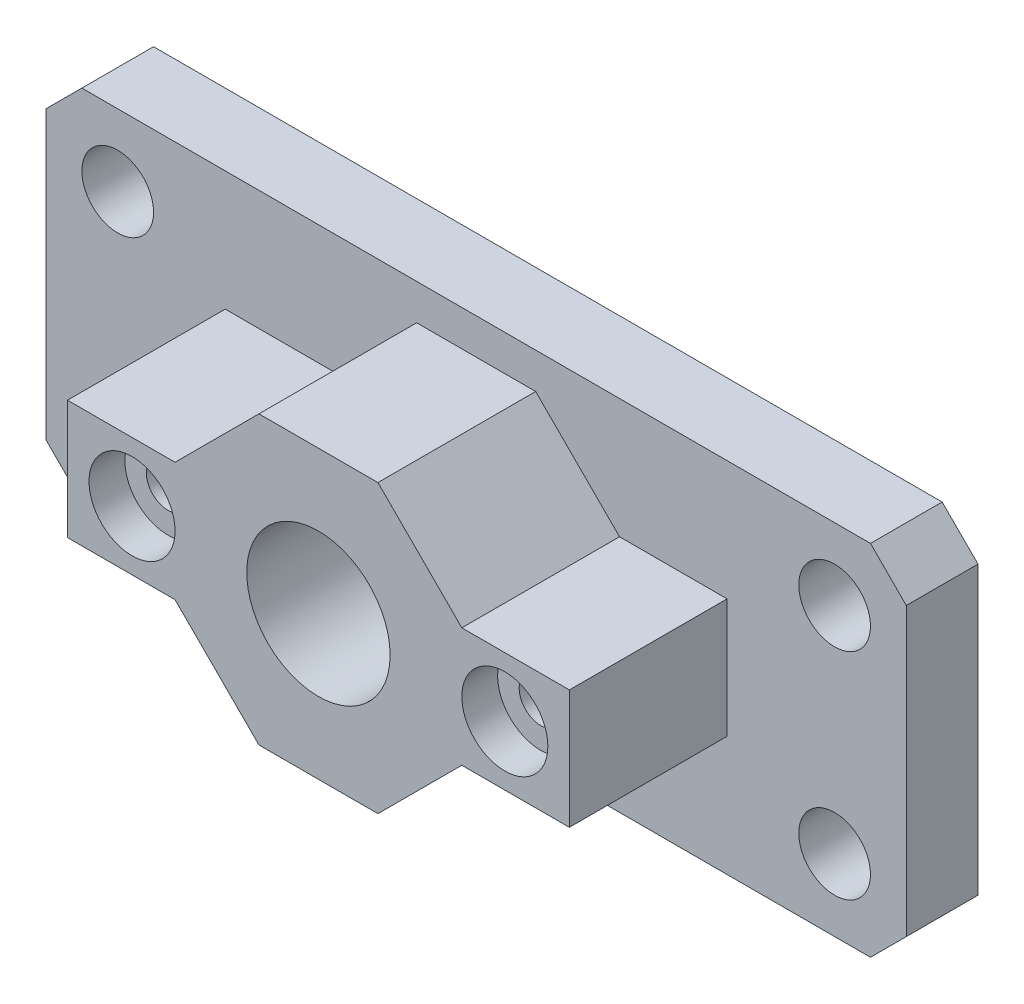
ISO-10303-21;
HEADER;
FILE_DESCRIPTION(('STEP AP214'),'2;1');
FILE_NAME('part.step','',(''),(''),'','','');
FILE_SCHEMA(('AUTOMOTIVE_DESIGN { 1 0 10303 214 1 1 1 1 }'));
ENDSEC;
DATA;
#1=APPLICATION_CONTEXT('core data for automotive mechanical design processes');
#2=APPLICATION_PROTOCOL_DEFINITION('international standard','automotive_design',2000,#1);
#3=PRODUCT_CONTEXT('',#1,'mechanical');
#4=PRODUCT('Part','Part','',(#3));
#5=PRODUCT_RELATED_PRODUCT_CATEGORY('part','',(#4));
#6=PRODUCT_DEFINITION_FORMATION('','',#4);
#7=PRODUCT_DEFINITION_CONTEXT('part definition',#1,'design');
#8=PRODUCT_DEFINITION('design','',#6,#7);
#9=PRODUCT_DEFINITION_SHAPE('','',#8);
#10=(LENGTH_UNIT() NAMED_UNIT(*) SI_UNIT(.MILLI.,.METRE.));
#11=(NAMED_UNIT(*) PLANE_ANGLE_UNIT() SI_UNIT($,.RADIAN.));
#12=(NAMED_UNIT(*) SI_UNIT($,.STERADIAN.) SOLID_ANGLE_UNIT());
#13=UNCERTAINTY_MEASURE_WITH_UNIT(LENGTH_MEASURE(1.E-05),#10,'distance_accuracy_value','');
#14=(GEOMETRIC_REPRESENTATION_CONTEXT(3) GLOBAL_UNCERTAINTY_ASSIGNED_CONTEXT((#13)) GLOBAL_UNIT_ASSIGNED_CONTEXT((#10,
#11,#12)) REPRESENTATION_CONTEXT('',''));
#15=CARTESIAN_POINT('',(0.,0.,0.));
#16=DIRECTION('',(0.,0.,1.));
#17=DIRECTION('',(1.,0.,0.));
#18=AXIS2_PLACEMENT_3D('',#15,#16,#17);
#19=CARTESIAN_POINT('',(60.,25.,10.));
#20=DIRECTION('',(-1.,0.,0.));
#21=DIRECTION('',(0.,-1.,0.));
#22=AXIS2_PLACEMENT_3D('',#19,#20,#21);
#23=PLANE('',#22);
#24=DIRECTION('',(0.,1.,0.));
#25=VECTOR('',#24,1.);
#26=CARTESIAN_POINT('',(60.,25.,10.));
#27=LINE('',#26,#25);
#28=CARTESIAN_POINT('',(60.,-20.,10.));
#29=VERTEX_POINT('',#28);
#30=CARTESIAN_POINT('',(60.,20.,10.));
#31=VERTEX_POINT('',#30);
#32=EDGE_CURVE('E216',#29,#31,#27,.T.);
#33=ORIENTED_EDGE('',*,*,#32,.F.);
#34=DIRECTION('',(0.,0.,-1.));
#35=VECTOR('',#34,1.);
#36=CARTESIAN_POINT('',(60.,-20.,10.));
#37=LINE('',#36,#35);
#38=CARTESIAN_POINT('',(60.,-20.,0.));
#39=VERTEX_POINT('',#38);
#40=EDGE_CURVE('E249',#29,#39,#37,.T.);
#41=ORIENTED_EDGE('',*,*,#40,.T.);
#42=DIRECTION('',(0.,1.,0.));
#43=VECTOR('',#42,1.);
#44=CARTESIAN_POINT('',(60.,25.,0.));
#45=LINE('',#44,#43);
#46=CARTESIAN_POINT('',(60.,20.,0.));
#47=VERTEX_POINT('',#46);
#48=EDGE_CURVE('E210',#39,#47,#45,.T.);
#49=ORIENTED_EDGE('',*,*,#48,.T.);
#50=DIRECTION('',(0.,0.,1.));
#51=VECTOR('',#50,1.);
#52=CARTESIAN_POINT('',(60.,20.,10.));
#53=LINE('',#52,#51);
#54=EDGE_CURVE('E227',#47,#31,#53,.T.);
#55=ORIENTED_EDGE('',*,*,#54,.T.);
#56=EDGE_LOOP('',(#33,#41,#49,#55));
#57=FACE_BOUND('',#56,.T.);
#58=ADVANCED_FACE('F41',(#57),#23,.F.);
#59=CARTESIAN_POINT('',(-60.,25.,10.));
#60=DIRECTION('',(0.,-1.,0.));
#61=DIRECTION('',(0.,0.,-1.));
#62=AXIS2_PLACEMENT_3D('',#59,#60,#61);
#63=PLANE('',#62);
#64=DIRECTION('',(-1.,0.,0.));
#65=VECTOR('',#64,1.);
#66=CARTESIAN_POINT('',(-60.,25.,0.));
#67=LINE('',#66,#65);
#68=CARTESIAN_POINT('',(55.,25.,0.));
#69=VERTEX_POINT('',#68);
#70=CARTESIAN_POINT('',(-55.,25.,0.));
#71=VERTEX_POINT('',#70);
#72=EDGE_CURVE('E209',#69,#71,#67,.T.);
#73=ORIENTED_EDGE('',*,*,#72,.T.);
#74=DIRECTION('',(0.,0.,1.));
#75=VECTOR('',#74,1.);
#76=CARTESIAN_POINT('',(-55.,25.,10.));
#77=LINE('',#76,#75);
#78=CARTESIAN_POINT('',(-55.,25.,10.));
#79=VERTEX_POINT('',#78);
#80=EDGE_CURVE('E11',#71,#79,#77,.T.);
#81=ORIENTED_EDGE('',*,*,#80,.T.);
#82=DIRECTION('',(-1.,0.,0.));
#83=VECTOR('',#82,1.);
#84=CARTESIAN_POINT('',(-60.,25.,10.));
#85=LINE('',#84,#83);
#86=CARTESIAN_POINT('',(55.,25.,10.));
#87=VERTEX_POINT('',#86);
#88=EDGE_CURVE('E218',#87,#79,#85,.T.);
#89=ORIENTED_EDGE('',*,*,#88,.F.);
#90=DIRECTION('',(0.,0.,-1.));
#91=VECTOR('',#90,1.);
#92=CARTESIAN_POINT('',(55.,25.,10.));
#93=LINE('',#92,#91);
#94=EDGE_CURVE('E49',#87,#69,#93,.T.);
#95=ORIENTED_EDGE('',*,*,#94,.T.);
#96=EDGE_LOOP('',(#73,#81,#89,#95));
#97=FACE_BOUND('',#96,.T.);
#98=ADVANCED_FACE('F278',(#97),#63,.F.);
#99=CARTESIAN_POINT('',(-60.,25.,10.));
#100=DIRECTION('',(1.,0.,0.));
#101=DIRECTION('',(0.,1.,0.));
#102=AXIS2_PLACEMENT_3D('',#99,#100,#101);
#103=PLANE('',#102);
#104=DIRECTION('',(0.,-1.,0.));
#105=VECTOR('',#104,1.);
#106=CARTESIAN_POINT('',(-60.,25.,0.));
#107=LINE('',#106,#105);
#108=CARTESIAN_POINT('',(-60.,20.,0.));
#109=VERTEX_POINT('',#108);
#110=CARTESIAN_POINT('',(-60.,-20.,0.));
#111=VERTEX_POINT('',#110);
#112=EDGE_CURVE('E228',#109,#111,#107,.T.);
#113=ORIENTED_EDGE('',*,*,#112,.T.);
#114=DIRECTION('',(0.,0.,1.));
#115=VECTOR('',#114,1.);
#116=CARTESIAN_POINT('',(-60.,-20.,10.));
#117=LINE('',#116,#115);
#118=CARTESIAN_POINT('',(-60.,-20.,10.));
#119=VERTEX_POINT('',#118);
#120=EDGE_CURVE('E60',#111,#119,#117,.T.);
#121=ORIENTED_EDGE('',*,*,#120,.T.);
#122=DIRECTION('',(0.,-1.,0.));
#123=VECTOR('',#122,1.);
#124=CARTESIAN_POINT('',(-60.,25.,10.));
#125=LINE('',#124,#123);
#126=CARTESIAN_POINT('',(-60.,20.,10.));
#127=VERTEX_POINT('',#126);
#128=EDGE_CURVE('E225',#127,#119,#125,.T.);
#129=ORIENTED_EDGE('',*,*,#128,.F.);
#130=DIRECTION('',(0.,0.,-1.));
#131=VECTOR('',#130,1.);
#132=CARTESIAN_POINT('',(-60.,20.,10.));
#133=LINE('',#132,#131);
#134=EDGE_CURVE('E275',#127,#109,#133,.T.);
#135=ORIENTED_EDGE('',*,*,#134,.T.);
#136=EDGE_LOOP('',(#113,#121,#129,#135));
#137=FACE_BOUND('',#136,.T.);
#138=ADVANCED_FACE('F292',(#137),#103,.F.);
#139=CARTESIAN_POINT('',(-60.,-25.,10.));
#140=DIRECTION('',(0.,1.,0.));
#141=DIRECTION('',(0.,0.,1.));
#142=AXIS2_PLACEMENT_3D('',#139,#140,#141);
#143=PLANE('',#142);
#144=DIRECTION('',(1.,0.,0.));
#145=VECTOR('',#144,1.);
#146=CARTESIAN_POINT('',(-60.,-25.,0.));
#147=LINE('',#146,#145);
#148=CARTESIAN_POINT('',(-55.,-25.,0.));
#149=VERTEX_POINT('',#148);
#150=CARTESIAN_POINT('',(55.,-25.,0.));
#151=VERTEX_POINT('',#150);
#152=EDGE_CURVE('E219',#149,#151,#147,.T.);
#153=ORIENTED_EDGE('',*,*,#152,.T.);
#154=DIRECTION('',(0.,0.,1.));
#155=VECTOR('',#154,1.);
#156=CARTESIAN_POINT('',(55.,-25.,10.));
#157=LINE('',#156,#155);
#158=CARTESIAN_POINT('',(55.,-25.,10.));
#159=VERTEX_POINT('',#158);
#160=EDGE_CURVE('E263',#151,#159,#157,.T.);
#161=ORIENTED_EDGE('',*,*,#160,.T.);
#162=DIRECTION('',(1.,0.,0.));
#163=VECTOR('',#162,1.);
#164=CARTESIAN_POINT('',(-60.,-25.,10.));
#165=LINE('',#164,#163);
#166=CARTESIAN_POINT('',(-55.,-25.,10.));
#167=VERTEX_POINT('',#166);
#168=EDGE_CURVE('E221',#167,#159,#165,.T.);
#169=ORIENTED_EDGE('',*,*,#168,.F.);
#170=DIRECTION('',(0.,0.,-1.));
#171=VECTOR('',#170,1.);
#172=CARTESIAN_POINT('',(-55.,-25.,10.));
#173=LINE('',#172,#171);
#174=EDGE_CURVE('E257',#167,#149,#173,.T.);
#175=ORIENTED_EDGE('',*,*,#174,.T.);
#176=EDGE_LOOP('',(#153,#161,#169,#175));
#177=FACE_BOUND('',#176,.T.);
#178=ADVANCED_FACE('F298',(#177),#143,.F.);
#179=CARTESIAN_POINT('',(0.,0.,10.));
#180=DIRECTION('',(0.,0.,1.));
#181=DIRECTION('',(1.,0.,0.));
#182=AXIS2_PLACEMENT_3D('',#179,#180,#181);
#183=PLANE('',#182);
#184=CARTESIAN_POINT('',(50.,-15.,10.));
#185=DIRECTION('',(0.,0.,1.));
#186=DIRECTION('',(1.,0.,0.));
#187=AXIS2_PLACEMENT_3D('',#184,#185,#186);
#188=CIRCLE('',#187,5.);
#189=CARTESIAN_POINT('',(55.,-15.,10.));
#190=VERTEX_POINT('',#189);
#191=EDGE_CURVE('E643',#190,#190,#188,.T.);
#192=ORIENTED_EDGE('',*,*,#191,.F.);
#193=EDGE_LOOP('',(#192));
#194=FACE_BOUND('',#193,.T.);
#195=CARTESIAN_POINT('',(-50.,15.,10.));
#196=DIRECTION('',(0.,0.,1.));
#197=DIRECTION('',(1.,0.,0.));
#198=AXIS2_PLACEMENT_3D('',#195,#196,#197);
#199=CIRCLE('',#198,5.);
#200=CARTESIAN_POINT('',(-45.,15.,10.));
#201=VERTEX_POINT('',#200);
#202=EDGE_CURVE('E642',#201,#201,#199,.T.);
#203=ORIENTED_EDGE('',*,*,#202,.F.);
#204=EDGE_LOOP('',(#203));
#205=FACE_BOUND('',#204,.T.);
#206=CARTESIAN_POINT('',(-50.,-15.,10.));
#207=DIRECTION('',(0.,0.,1.));
#208=DIRECTION('',(1.,0.,0.));
#209=AXIS2_PLACEMENT_3D('',#206,#207,#208);
#210=CIRCLE('',#209,5.);
#211=CARTESIAN_POINT('',(-45.,-15.,10.));
#212=VERTEX_POINT('',#211);
#213=EDGE_CURVE('E647',#212,#212,#210,.T.);
#214=ORIENTED_EDGE('',*,*,#213,.F.);
#215=EDGE_LOOP('',(#214));
#216=FACE_BOUND('',#215,.T.);
#217=CARTESIAN_POINT('',(50.,15.,10.));
#218=DIRECTION('',(0.,0.,1.));
#219=DIRECTION('',(1.,0.,0.));
#220=AXIS2_PLACEMENT_3D('',#217,#218,#219);
#221=CIRCLE('',#220,5.);
#222=CARTESIAN_POINT('',(55.,15.,10.));
#223=VERTEX_POINT('',#222);
#224=EDGE_CURVE('E236',#223,#223,#221,.T.);
#225=ORIENTED_EDGE('',*,*,#224,.F.);
#226=EDGE_LOOP('',(#225));
#227=FACE_BOUND('',#226,.T.);
#228=DIRECTION('',(-1.,0.,0.));
#229=VECTOR('',#228,1.);
#230=CARTESIAN_POINT('',(8.3,20.,10.));
#231=LINE('',#230,#229);
#232=CARTESIAN_POINT('',(8.3,20.,10.));
#233=VERTEX_POINT('',#232);
#234=CARTESIAN_POINT('',(-8.3,20.,10.));
#235=VERTEX_POINT('',#234);
#236=EDGE_CURVE('E206',#233,#235,#231,.T.);
#237=ORIENTED_EDGE('',*,*,#236,.F.);
#238=DIRECTION('',(-0.707106781186548,0.707106781186547,0.));
#239=VECTOR('',#238,1.);
#240=CARTESIAN_POINT('',(20.,8.3,10.));
#241=LINE('',#240,#239);
#242=CARTESIAN_POINT('',(20.,8.3,10.));
#243=VERTEX_POINT('',#242);
#244=EDGE_CURVE('E201',#243,#233,#241,.T.);
#245=ORIENTED_EDGE('',*,*,#244,.F.);
#246=DIRECTION('',(1.,0.,0.));
#247=VECTOR('',#246,1.);
#248=CARTESIAN_POINT('',(20.,8.3,10.));
#249=LINE('',#248,#247);
#250=CARTESIAN_POINT('',(35.,8.3,10.));
#251=VERTEX_POINT('',#250);
#252=EDGE_CURVE('E662',#243,#251,#249,.T.);
#253=ORIENTED_EDGE('',*,*,#252,.T.);
#254=DIRECTION('',(0.,-1.,0.));
#255=VECTOR('',#254,1.);
#256=CARTESIAN_POINT('',(35.,8.3,10.));
#257=LINE('',#256,#255);
#258=CARTESIAN_POINT('',(35.,-8.3,10.));
#259=VERTEX_POINT('',#258);
#260=EDGE_CURVE('E717',#251,#259,#257,.T.);
#261=ORIENTED_EDGE('',*,*,#260,.T.);
#262=DIRECTION('',(1.,0.,0.));
#263=VECTOR('',#262,1.);
#264=CARTESIAN_POINT('',(20.,-8.3,10.));
#265=LINE('',#264,#263);
#266=CARTESIAN_POINT('',(20.,-8.3,10.));
#267=VERTEX_POINT('',#266);
#268=EDGE_CURVE('E712',#267,#259,#265,.T.);
#269=ORIENTED_EDGE('',*,*,#268,.F.);
#270=DIRECTION('',(0.707106781186548,0.707106781186547,0.));
#271=VECTOR('',#270,1.);
#272=CARTESIAN_POINT('',(8.3,-20.,10.));
#273=LINE('',#272,#271);
#274=CARTESIAN_POINT('',(8.3,-20.,10.));
#275=VERTEX_POINT('',#274);
#276=EDGE_CURVE('E709',#275,#267,#273,.T.);
#277=ORIENTED_EDGE('',*,*,#276,.F.);
#278=DIRECTION('',(1.,0.,0.));
#279=VECTOR('',#278,1.);
#280=CARTESIAN_POINT('',(-8.3,-20.,10.));
#281=LINE('',#280,#279);
#282=CARTESIAN_POINT('',(-8.3,-20.,10.));
#283=VERTEX_POINT('',#282);
#284=EDGE_CURVE('E710',#283,#275,#281,.T.);
#285=ORIENTED_EDGE('',*,*,#284,.F.);
#286=DIRECTION('',(0.707106781186548,-0.707106781186548,0.));
#287=VECTOR('',#286,1.);
#288=CARTESIAN_POINT('',(-20.,-8.3,10.));
#289=LINE('',#288,#287);
#290=CARTESIAN_POINT('',(-20.,-8.3,10.));
#291=VERTEX_POINT('',#290);
#292=EDGE_CURVE('E702',#291,#283,#289,.T.);
#293=ORIENTED_EDGE('',*,*,#292,.F.);
#294=DIRECTION('',(1.,0.,0.));
#295=VECTOR('',#294,1.);
#296=CARTESIAN_POINT('',(-35.,-8.3,10.));
#297=LINE('',#296,#295);
#298=CARTESIAN_POINT('',(-35.,-8.3,10.));
#299=VERTEX_POINT('',#298);
#300=EDGE_CURVE('E696',#299,#291,#297,.T.);
#301=ORIENTED_EDGE('',*,*,#300,.F.);
#302=DIRECTION('',(0.,-1.,0.));
#303=VECTOR('',#302,1.);
#304=CARTESIAN_POINT('',(-35.,8.3,10.));
#305=LINE('',#304,#303);
#306=CARTESIAN_POINT('',(-35.,8.3,10.));
#307=VERTEX_POINT('',#306);
#308=EDGE_CURVE('E695',#307,#299,#305,.T.);
#309=ORIENTED_EDGE('',*,*,#308,.F.);
#310=DIRECTION('',(1.,0.,0.));
#311=VECTOR('',#310,1.);
#312=CARTESIAN_POINT('',(-35.,8.3,10.));
#313=LINE('',#312,#311);
#314=CARTESIAN_POINT('',(-20.,8.3,10.));
#315=VERTEX_POINT('',#314);
#316=EDGE_CURVE('E698',#307,#315,#313,.T.);
#317=ORIENTED_EDGE('',*,*,#316,.T.);
#318=DIRECTION('',(-0.707106781186547,-0.707106781186548,0.));
#319=VECTOR('',#318,1.);
#320=CARTESIAN_POINT('',(-8.3,20.,10.));
#321=LINE('',#320,#319);
#322=EDGE_CURVE('E654',#235,#315,#321,.T.);
#323=ORIENTED_EDGE('',*,*,#322,.F.);
#324=EDGE_LOOP('',(#237,#245,#253,#261,#269,#277,#285,#293,#301,#309,#317,#323));
#325=FACE_BOUND('',#324,.T.);
#326=ORIENTED_EDGE('',*,*,#168,.T.);
#327=DIRECTION('',(-0.707106781186549,-0.707106781186547,0.));
#328=VECTOR('',#327,1.);
#329=CARTESIAN_POINT('',(39.9999999999999,-40.,10.));
#330=LINE('',#329,#328);
#331=EDGE_CURVE('E269',#159,#29,#330,.F.);
#332=ORIENTED_EDGE('',*,*,#331,.T.);
#333=ORIENTED_EDGE('',*,*,#32,.T.);
#334=DIRECTION('',(0.707106781186547,-0.707106781186549,0.));
#335=VECTOR('',#334,1.);
#336=CARTESIAN_POINT('',(40.0000000000001,40.,10.));
#337=LINE('',#336,#335);
#338=EDGE_CURVE('E264',#31,#87,#337,.F.);
#339=ORIENTED_EDGE('',*,*,#338,.T.);
#340=ORIENTED_EDGE('',*,*,#88,.T.);
#341=DIRECTION('',(0.707106781186549,0.707106781186547,0.));
#342=VECTOR('',#341,1.);
#343=CARTESIAN_POINT('',(-39.9999999999999,40.,10.));
#344=LINE('',#343,#342);
#345=EDGE_CURVE('E61',#79,#127,#344,.F.);
#346=ORIENTED_EDGE('',*,*,#345,.T.);
#347=ORIENTED_EDGE('',*,*,#128,.T.);
#348=DIRECTION('',(-0.707106781186547,0.707106781186549,0.));
#349=VECTOR('',#348,1.);
#350=CARTESIAN_POINT('',(-40.0000000000001,-40.,10.));
#351=LINE('',#350,#349);
#352=EDGE_CURVE('E268',#119,#167,#351,.F.);
#353=ORIENTED_EDGE('',*,*,#352,.T.);
#354=EDGE_LOOP('',(#326,#332,#333,#339,#340,#346,#347,#353));
#355=FACE_BOUND('',#354,.T.);
#356=ADVANCED_FACE('F291',(#194,#205,#216,#227,#325,#355),#183,.T.);
#357=CARTESIAN_POINT('',(0.,0.,0.));
#358=DIRECTION('',(0.,0.,1.));
#359=DIRECTION('',(1.,0.,0.));
#360=AXIS2_PLACEMENT_3D('',#357,#358,#359);
#361=PLANE('',#360);
#362=CARTESIAN_POINT('',(50.,-15.,0.));
#363=DIRECTION('',(0.,0.,1.));
#364=DIRECTION('',(1.,0.,0.));
#365=AXIS2_PLACEMENT_3D('',#362,#363,#364);
#366=CIRCLE('',#365,5.);
#367=CARTESIAN_POINT('',(55.,-15.,0.));
#368=VERTEX_POINT('',#367);
#369=EDGE_CURVE('E241',#368,#368,#366,.T.);
#370=ORIENTED_EDGE('',*,*,#369,.T.);
#371=EDGE_LOOP('',(#370));
#372=FACE_BOUND('',#371,.T.);
#373=CARTESIAN_POINT('',(-50.,15.,0.));
#374=DIRECTION('',(0.,0.,1.));
#375=DIRECTION('',(1.,0.,0.));
#376=AXIS2_PLACEMENT_3D('',#373,#374,#375);
#377=CIRCLE('',#376,5.);
#378=CARTESIAN_POINT('',(-45.,15.,0.));
#379=VERTEX_POINT('',#378);
#380=EDGE_CURVE('E242',#379,#379,#377,.T.);
#381=ORIENTED_EDGE('',*,*,#380,.T.);
#382=EDGE_LOOP('',(#381));
#383=FACE_BOUND('',#382,.T.);
#384=CARTESIAN_POINT('',(-50.,-15.,0.));
#385=DIRECTION('',(0.,0.,1.));
#386=DIRECTION('',(1.,0.,0.));
#387=AXIS2_PLACEMENT_3D('',#384,#385,#386);
#388=CIRCLE('',#387,5.);
#389=CARTESIAN_POINT('',(-45.,-15.,0.));
#390=VERTEX_POINT('',#389);
#391=EDGE_CURVE('E240',#390,#390,#388,.T.);
#392=ORIENTED_EDGE('',*,*,#391,.T.);
#393=EDGE_LOOP('',(#392));
#394=FACE_BOUND('',#393,.T.);
#395=CARTESIAN_POINT('',(50.,15.,0.));
#396=DIRECTION('',(0.,0.,1.));
#397=DIRECTION('',(1.,0.,0.));
#398=AXIS2_PLACEMENT_3D('',#395,#396,#397);
#399=CIRCLE('',#398,5.);
#400=CARTESIAN_POINT('',(55.,15.,0.));
#401=VERTEX_POINT('',#400);
#402=EDGE_CURVE('E234',#401,#401,#399,.T.);
#403=ORIENTED_EDGE('',*,*,#402,.T.);
#404=EDGE_LOOP('',(#403));
#405=FACE_BOUND('',#404,.T.);
#406=ORIENTED_EDGE('',*,*,#48,.F.);
#407=DIRECTION('',(0.707106781186549,0.707106781186547,0.));
#408=VECTOR('',#407,1.);
#409=CARTESIAN_POINT('',(60.,-20.,0.));
#410=LINE('',#409,#408);
#411=EDGE_CURVE('E256',#39,#151,#410,.F.);
#412=ORIENTED_EDGE('',*,*,#411,.T.);
#413=ORIENTED_EDGE('',*,*,#152,.F.);
#414=DIRECTION('',(0.707106781186547,-0.707106781186549,0.));
#415=VECTOR('',#414,1.);
#416=CARTESIAN_POINT('',(-55.,-25.,0.));
#417=LINE('',#416,#415);
#418=EDGE_CURVE('E258',#149,#111,#417,.F.);
#419=ORIENTED_EDGE('',*,*,#418,.T.);
#420=ORIENTED_EDGE('',*,*,#112,.F.);
#421=DIRECTION('',(-0.707106781186549,-0.707106781186547,0.));
#422=VECTOR('',#421,1.);
#423=CARTESIAN_POINT('',(-60.,20.,0.));
#424=LINE('',#423,#422);
#425=EDGE_CURVE('E255',#109,#71,#424,.F.);
#426=ORIENTED_EDGE('',*,*,#425,.T.);
#427=ORIENTED_EDGE('',*,*,#72,.F.);
#428=DIRECTION('',(-0.707106781186547,0.707106781186549,0.));
#429=VECTOR('',#428,1.);
#430=CARTESIAN_POINT('',(55.,25.,0.));
#431=LINE('',#430,#429);
#432=EDGE_CURVE('E252',#69,#47,#431,.F.);
#433=ORIENTED_EDGE('',*,*,#432,.T.);
#434=EDGE_LOOP('',(#406,#412,#413,#419,#420,#426,#427,#433));
#435=FACE_BOUND('',#434,.T.);
#436=ADVANCED_FACE('F287',(#372,#383,#394,#405,#435),#361,.F.);
#437=CARTESIAN_POINT('',(8.3,20.,32.));
#438=DIRECTION('',(0.,-1.,0.));
#439=DIRECTION('',(1.,0.,0.));
#440=AXIS2_PLACEMENT_3D('',#437,#438,#439);
#441=PLANE('',#440);
#442=ORIENTED_EDGE('',*,*,#236,.T.);
#443=DIRECTION('',(0.,0.,-1.));
#444=VECTOR('',#443,1.);
#445=CARTESIAN_POINT('',(-8.3,20.,32.));
#446=LINE('',#445,#444);
#447=CARTESIAN_POINT('',(-8.3,20.,32.));
#448=VERTEX_POINT('',#447);
#449=EDGE_CURVE('E183',#448,#235,#446,.T.);
#450=ORIENTED_EDGE('',*,*,#449,.F.);
#451=DIRECTION('',(-1.,0.,0.));
#452=VECTOR('',#451,1.);
#453=CARTESIAN_POINT('',(8.3,20.,32.));
#454=LINE('',#453,#452);
#455=CARTESIAN_POINT('',(8.3,20.,32.));
#456=VERTEX_POINT('',#455);
#457=EDGE_CURVE('E193',#456,#448,#454,.T.);
#458=ORIENTED_EDGE('',*,*,#457,.F.);
#459=DIRECTION('',(0.,0.,-1.));
#460=VECTOR('',#459,1.);
#461=CARTESIAN_POINT('',(8.3,20.,32.));
#462=LINE('',#461,#460);
#463=EDGE_CURVE('E657',#456,#233,#462,.T.);
#464=ORIENTED_EDGE('',*,*,#463,.T.);
#465=EDGE_LOOP('',(#442,#450,#458,#464));
#466=FACE_BOUND('',#465,.T.);
#467=ADVANCED_FACE('F202',(#466),#441,.F.);
#468=CARTESIAN_POINT('',(-8.3,20.,32.));
#469=DIRECTION('',(0.707106781186548,-0.707106781186547,0.));
#470=DIRECTION('',(0.707106781186547,0.707106781186548,0.));
#471=AXIS2_PLACEMENT_3D('',#468,#469,#470);
#472=PLANE('',#471);
#473=ORIENTED_EDGE('',*,*,#322,.T.);
#474=DIRECTION('',(0.,0.,-1.));
#475=VECTOR('',#474,1.);
#476=CARTESIAN_POINT('',(-20.,8.3,32.));
#477=LINE('',#476,#475);
#478=CARTESIAN_POINT('',(-20.,8.3,32.));
#479=VERTEX_POINT('',#478);
#480=EDGE_CURVE('E190',#479,#315,#477,.T.);
#481=ORIENTED_EDGE('',*,*,#480,.F.);
#482=DIRECTION('',(-0.707106781186547,-0.707106781186548,0.));
#483=VECTOR('',#482,1.);
#484=CARTESIAN_POINT('',(-8.3,20.,32.));
#485=LINE('',#484,#483);
#486=EDGE_CURVE('E176',#448,#479,#485,.T.);
#487=ORIENTED_EDGE('',*,*,#486,.F.);
#488=ORIENTED_EDGE('',*,*,#449,.T.);
#489=EDGE_LOOP('',(#473,#481,#487,#488));
#490=FACE_BOUND('',#489,.T.);
#491=ADVANCED_FACE('F181',(#490),#472,.F.);
#492=CARTESIAN_POINT('',(-35.,8.3,32.));
#493=DIRECTION('',(0.,1.,0.));
#494=DIRECTION('',(0.,0.,1.));
#495=AXIS2_PLACEMENT_3D('',#492,#493,#494);
#496=PLANE('',#495);
#497=ORIENTED_EDGE('',*,*,#316,.F.);
#498=DIRECTION('',(0.,0.,-1.));
#499=VECTOR('',#498,1.);
#500=CARTESIAN_POINT('',(-35.,8.3,32.));
#501=LINE('',#500,#499);
#502=CARTESIAN_POINT('',(-35.,8.3,32.));
#503=VERTEX_POINT('',#502);
#504=EDGE_CURVE('E215',#503,#307,#501,.T.);
#505=ORIENTED_EDGE('',*,*,#504,.F.);
#506=DIRECTION('',(1.,0.,0.));
#507=VECTOR('',#506,1.);
#508=CARTESIAN_POINT('',(-35.,8.3,32.));
#509=LINE('',#508,#507);
#510=EDGE_CURVE('E195',#503,#479,#509,.T.);
#511=ORIENTED_EDGE('',*,*,#510,.T.);
#512=ORIENTED_EDGE('',*,*,#480,.T.);
#513=EDGE_LOOP('',(#497,#505,#511,#512));
#514=FACE_BOUND('',#513,.T.);
#515=ADVANCED_FACE('F568',(#514),#496,.T.);
#516=CARTESIAN_POINT('',(-35.,8.3,32.));
#517=DIRECTION('',(1.,0.,0.));
#518=DIRECTION('',(0.,0.,-1.));
#519=AXIS2_PLACEMENT_3D('',#516,#517,#518);
#520=PLANE('',#519);
#521=ORIENTED_EDGE('',*,*,#308,.T.);
#522=DIRECTION('',(0.,0.,-1.));
#523=VECTOR('',#522,1.);
#524=CARTESIAN_POINT('',(-35.,-8.3,32.));
#525=LINE('',#524,#523);
#526=CARTESIAN_POINT('',(-35.,-8.3,32.));
#527=VERTEX_POINT('',#526);
#528=EDGE_CURVE('E690',#527,#299,#525,.T.);
#529=ORIENTED_EDGE('',*,*,#528,.F.);
#530=DIRECTION('',(0.,-1.,0.));
#531=VECTOR('',#530,1.);
#532=CARTESIAN_POINT('',(-35.,8.3,32.));
#533=LINE('',#532,#531);
#534=EDGE_CURVE('E694',#503,#527,#533,.T.);
#535=ORIENTED_EDGE('',*,*,#534,.F.);
#536=ORIENTED_EDGE('',*,*,#504,.T.);
#537=EDGE_LOOP('',(#521,#529,#535,#536));
#538=FACE_BOUND('',#537,.T.);
#539=ADVANCED_FACE('F562',(#538),#520,.F.);
#540=CARTESIAN_POINT('',(-35.,-8.3,32.));
#541=DIRECTION('',(0.,1.,0.));
#542=DIRECTION('',(0.,0.,1.));
#543=AXIS2_PLACEMENT_3D('',#540,#541,#542);
#544=PLANE('',#543);
#545=ORIENTED_EDGE('',*,*,#300,.T.);
#546=DIRECTION('',(0.,0.,-1.));
#547=VECTOR('',#546,1.);
#548=CARTESIAN_POINT('',(-20.,-8.3,32.));
#549=LINE('',#548,#547);
#550=CARTESIAN_POINT('',(-20.,-8.3,32.));
#551=VERTEX_POINT('',#550);
#552=EDGE_CURVE('E681',#551,#291,#549,.T.);
#553=ORIENTED_EDGE('',*,*,#552,.F.);
#554=DIRECTION('',(1.,0.,0.));
#555=VECTOR('',#554,1.);
#556=CARTESIAN_POINT('',(-35.,-8.3,32.));
#557=LINE('',#556,#555);
#558=EDGE_CURVE('E733',#527,#551,#557,.T.);
#559=ORIENTED_EDGE('',*,*,#558,.F.);
#560=ORIENTED_EDGE('',*,*,#528,.T.);
#561=EDGE_LOOP('',(#545,#553,#559,#560));
#562=FACE_BOUND('',#561,.T.);
#563=ADVANCED_FACE('F555',(#562),#544,.F.);
#564=CARTESIAN_POINT('',(-20.,-8.3,32.));
#565=DIRECTION('',(0.707106781186548,0.707106781186548,0.));
#566=DIRECTION('',(-0.707106781186548,0.707106781186548,0.));
#567=AXIS2_PLACEMENT_3D('',#564,#565,#566);
#568=PLANE('',#567);
#569=ORIENTED_EDGE('',*,*,#292,.T.);
#570=DIRECTION('',(0.,0.,-1.));
#571=VECTOR('',#570,1.);
#572=CARTESIAN_POINT('',(-8.3,-20.,32.));
#573=LINE('',#572,#571);
#574=CARTESIAN_POINT('',(-8.3,-20.,32.));
#575=VERTEX_POINT('',#574);
#576=EDGE_CURVE('E682',#575,#283,#573,.T.);
#577=ORIENTED_EDGE('',*,*,#576,.F.);
#578=DIRECTION('',(0.707106781186548,-0.707106781186548,0.));
#579=VECTOR('',#578,1.);
#580=CARTESIAN_POINT('',(-20.,-8.3,32.));
#581=LINE('',#580,#579);
#582=EDGE_CURVE('E731',#551,#575,#581,.T.);
#583=ORIENTED_EDGE('',*,*,#582,.F.);
#584=ORIENTED_EDGE('',*,*,#552,.T.);
#585=EDGE_LOOP('',(#569,#577,#583,#584));
#586=FACE_BOUND('',#585,.T.);
#587=ADVANCED_FACE('F543',(#586),#568,.F.);
#588=CARTESIAN_POINT('',(-8.3,-20.,32.));
#589=DIRECTION('',(0.,1.,0.));
#590=DIRECTION('',(-1.,0.,0.));
#591=AXIS2_PLACEMENT_3D('',#588,#589,#590);
#592=PLANE('',#591);
#593=ORIENTED_EDGE('',*,*,#284,.T.);
#594=DIRECTION('',(0.,0.,-1.));
#595=VECTOR('',#594,1.);
#596=CARTESIAN_POINT('',(8.3,-20.,32.));
#597=LINE('',#596,#595);
#598=CARTESIAN_POINT('',(8.3,-20.,32.));
#599=VERTEX_POINT('',#598);
#600=EDGE_CURVE('E676',#599,#275,#597,.T.);
#601=ORIENTED_EDGE('',*,*,#600,.F.);
#602=DIRECTION('',(1.,0.,0.));
#603=VECTOR('',#602,1.);
#604=CARTESIAN_POINT('',(-8.3,-20.,32.));
#605=LINE('',#604,#603);
#606=EDGE_CURVE('E729',#575,#599,#605,.T.);
#607=ORIENTED_EDGE('',*,*,#606,.F.);
#608=ORIENTED_EDGE('',*,*,#576,.T.);
#609=EDGE_LOOP('',(#593,#601,#607,#608));
#610=FACE_BOUND('',#609,.T.);
#611=ADVANCED_FACE('F534',(#610),#592,.F.);
#612=CARTESIAN_POINT('',(8.3,-20.,32.));
#613=DIRECTION('',(-0.707106781186547,0.707106781186548,0.));
#614=DIRECTION('',(-0.707106781186548,-0.707106781186547,0.));
#615=AXIS2_PLACEMENT_3D('',#612,#613,#614);
#616=PLANE('',#615);
#617=ORIENTED_EDGE('',*,*,#276,.T.);
#618=DIRECTION('',(0.,0.,-1.));
#619=VECTOR('',#618,1.);
#620=CARTESIAN_POINT('',(20.,-8.3,32.));
#621=LINE('',#620,#619);
#622=CARTESIAN_POINT('',(20.,-8.3,32.));
#623=VERTEX_POINT('',#622);
#624=EDGE_CURVE('E671',#623,#267,#621,.T.);
#625=ORIENTED_EDGE('',*,*,#624,.F.);
#626=DIRECTION('',(0.707106781186548,0.707106781186547,0.));
#627=VECTOR('',#626,1.);
#628=CARTESIAN_POINT('',(8.3,-20.,32.));
#629=LINE('',#628,#627);
#630=EDGE_CURVE('E730',#599,#623,#629,.T.);
#631=ORIENTED_EDGE('',*,*,#630,.F.);
#632=ORIENTED_EDGE('',*,*,#600,.T.);
#633=EDGE_LOOP('',(#617,#625,#631,#632));
#634=FACE_BOUND('',#633,.T.);
#635=ADVANCED_FACE('F521',(#634),#616,.F.);
#636=CARTESIAN_POINT('',(20.,-8.3,32.));
#637=DIRECTION('',(0.,1.,0.));
#638=DIRECTION('',(-1.,0.,0.));
#639=AXIS2_PLACEMENT_3D('',#636,#637,#638);
#640=PLANE('',#639);
#641=ORIENTED_EDGE('',*,*,#268,.T.);
#642=DIRECTION('',(0.,0.,-1.));
#643=VECTOR('',#642,1.);
#644=CARTESIAN_POINT('',(35.,-8.3,32.));
#645=LINE('',#644,#643);
#646=CARTESIAN_POINT('',(35.,-8.3,32.));
#647=VERTEX_POINT('',#646);
#648=EDGE_CURVE('E675',#647,#259,#645,.T.);
#649=ORIENTED_EDGE('',*,*,#648,.F.);
#650=DIRECTION('',(1.,0.,0.));
#651=VECTOR('',#650,1.);
#652=CARTESIAN_POINT('',(20.,-8.3,32.));
#653=LINE('',#652,#651);
#654=EDGE_CURVE('E743',#623,#647,#653,.T.);
#655=ORIENTED_EDGE('',*,*,#654,.F.);
#656=ORIENTED_EDGE('',*,*,#624,.T.);
#657=EDGE_LOOP('',(#641,#649,#655,#656));
#658=FACE_BOUND('',#657,.T.);
#659=ADVANCED_FACE('F517',(#658),#640,.F.);
#660=CARTESIAN_POINT('',(35.,8.3,32.));
#661=DIRECTION('',(1.,0.,0.));
#662=DIRECTION('',(0.,0.,-1.));
#663=AXIS2_PLACEMENT_3D('',#660,#661,#662);
#664=PLANE('',#663);
#665=ORIENTED_EDGE('',*,*,#260,.F.);
#666=DIRECTION('',(0.,0.,-1.));
#667=VECTOR('',#666,1.);
#668=CARTESIAN_POINT('',(35.,8.3,32.));
#669=LINE('',#668,#667);
#670=CARTESIAN_POINT('',(35.,8.3,32.));
#671=VERTEX_POINT('',#670);
#672=EDGE_CURVE('E661',#671,#251,#669,.T.);
#673=ORIENTED_EDGE('',*,*,#672,.F.);
#674=DIRECTION('',(0.,-1.,0.));
#675=VECTOR('',#674,1.);
#676=CARTESIAN_POINT('',(35.,8.3,32.));
#677=LINE('',#676,#675);
#678=EDGE_CURVE('E724',#671,#647,#677,.T.);
#679=ORIENTED_EDGE('',*,*,#678,.T.);
#680=ORIENTED_EDGE('',*,*,#648,.T.);
#681=EDGE_LOOP('',(#665,#673,#679,#680));
#682=FACE_BOUND('',#681,.T.);
#683=ADVANCED_FACE('F510',(#682),#664,.T.);
#684=CARTESIAN_POINT('',(20.,8.3,32.));
#685=DIRECTION('',(0.,1.,0.));
#686=DIRECTION('',(-1.,0.,0.));
#687=AXIS2_PLACEMENT_3D('',#684,#685,#686);
#688=PLANE('',#687);
#689=ORIENTED_EDGE('',*,*,#252,.F.);
#690=DIRECTION('',(0.,0.,-1.));
#691=VECTOR('',#690,1.);
#692=CARTESIAN_POINT('',(20.,8.3,32.));
#693=LINE('',#692,#691);
#694=CARTESIAN_POINT('',(20.,8.3,32.));
#695=VERTEX_POINT('',#694);
#696=EDGE_CURVE('E658',#695,#243,#693,.T.);
#697=ORIENTED_EDGE('',*,*,#696,.F.);
#698=DIRECTION('',(1.,0.,0.));
#699=VECTOR('',#698,1.);
#700=CARTESIAN_POINT('',(20.,8.3,32.));
#701=LINE('',#700,#699);
#702=EDGE_CURVE('E667',#695,#671,#701,.T.);
#703=ORIENTED_EDGE('',*,*,#702,.T.);
#704=ORIENTED_EDGE('',*,*,#672,.T.);
#705=EDGE_LOOP('',(#689,#697,#703,#704));
#706=FACE_BOUND('',#705,.T.);
#707=ADVANCED_FACE('F499',(#706),#688,.T.);
#708=CARTESIAN_POINT('',(20.,8.3,32.));
#709=DIRECTION('',(-0.707106781186547,-0.707106781186548,0.));
#710=DIRECTION('',(0.707106781186548,-0.707106781186547,0.));
#711=AXIS2_PLACEMENT_3D('',#708,#709,#710);
#712=PLANE('',#711);
#713=ORIENTED_EDGE('',*,*,#244,.T.);
#714=ORIENTED_EDGE('',*,*,#463,.F.);
#715=DIRECTION('',(-0.707106781186548,0.707106781186547,0.));
#716=VECTOR('',#715,1.);
#717=CARTESIAN_POINT('',(20.,8.3,32.));
#718=LINE('',#717,#716);
#719=EDGE_CURVE('E200',#695,#456,#718,.T.);
#720=ORIENTED_EDGE('',*,*,#719,.F.);
#721=ORIENTED_EDGE('',*,*,#696,.T.);
#722=EDGE_LOOP('',(#713,#714,#720,#721));
#723=FACE_BOUND('',#722,.T.);
#724=ADVANCED_FACE('F487',(#723),#712,.F.);
#725=CARTESIAN_POINT('',(0.,0.,32.));
#726=DIRECTION('',(0.,0.,1.));
#727=DIRECTION('',(1.,0.,0.));
#728=AXIS2_PLACEMENT_3D('',#725,#726,#727);
#729=PLANE('',#728);
#730=CARTESIAN_POINT('',(-26.,0.,32.));
#731=DIRECTION('',(0.,0.,1.));
#732=DIRECTION('',(1.,0.,0.));
#733=AXIS2_PLACEMENT_3D('',#730,#731,#732);
#734=CIRCLE('',#733,6.);
#735=CARTESIAN_POINT('',(-20.,0.,32.));
#736=VERTEX_POINT('',#735);
#737=EDGE_CURVE('E759',#736,#736,#734,.T.);
#738=ORIENTED_EDGE('',*,*,#737,.F.);
#739=EDGE_LOOP('',(#738));
#740=FACE_BOUND('',#739,.T.);
#741=CARTESIAN_POINT('',(26.,0.,32.));
#742=DIRECTION('',(0.,0.,1.));
#743=DIRECTION('',(1.,0.,0.));
#744=AXIS2_PLACEMENT_3D('',#741,#742,#743);
#745=CIRCLE('',#744,6.);
#746=CARTESIAN_POINT('',(32.,0.,32.));
#747=VERTEX_POINT('',#746);
#748=EDGE_CURVE('E756',#747,#747,#745,.T.);
#749=ORIENTED_EDGE('',*,*,#748,.F.);
#750=EDGE_LOOP('',(#749));
#751=FACE_BOUND('',#750,.T.);
#752=CARTESIAN_POINT('',(0.,0.,32.));
#753=DIRECTION('',(0.,0.,1.));
#754=DIRECTION('',(1.,0.,0.));
#755=AXIS2_PLACEMENT_3D('',#752,#753,#754);
#756=CIRCLE('',#755,10.);
#757=CARTESIAN_POINT('',(10.,0.,32.));
#758=VERTEX_POINT('',#757);
#759=EDGE_CURVE('E747',#758,#758,#756,.T.);
#760=ORIENTED_EDGE('',*,*,#759,.F.);
#761=EDGE_LOOP('',(#760));
#762=FACE_BOUND('',#761,.T.);
#763=ORIENTED_EDGE('',*,*,#457,.T.);
#764=ORIENTED_EDGE('',*,*,#486,.T.);
#765=ORIENTED_EDGE('',*,*,#510,.F.);
#766=ORIENTED_EDGE('',*,*,#534,.T.);
#767=ORIENTED_EDGE('',*,*,#558,.T.);
#768=ORIENTED_EDGE('',*,*,#582,.T.);
#769=ORIENTED_EDGE('',*,*,#606,.T.);
#770=ORIENTED_EDGE('',*,*,#630,.T.);
#771=ORIENTED_EDGE('',*,*,#654,.T.);
#772=ORIENTED_EDGE('',*,*,#678,.F.);
#773=ORIENTED_EDGE('',*,*,#702,.F.);
#774=ORIENTED_EDGE('',*,*,#719,.T.);
#775=EDGE_LOOP('',(#763,#764,#765,#766,#767,#768,#769,#770,#771,#772,#773,#774));
#776=FACE_BOUND('',#775,.T.);
#777=ADVANCED_FACE('F198',(#740,#751,#762,#776),#729,.T.);
#778=CARTESIAN_POINT('',(0.,0.,10.));
#779=DIRECTION('',(0.,0.,1.));
#780=DIRECTION('',(1.,0.,0.));
#781=AXIS2_PLACEMENT_3D('',#778,#779,#780);
#782=CYLINDRICAL_SURFACE('',#781,10.);
#783=CARTESIAN_POINT('',(0.,0.,10.));
#784=DIRECTION('',(0.,0.,1.));
#785=DIRECTION('',(1.,0.,0.));
#786=AXIS2_PLACEMENT_3D('',#783,#784,#785);
#787=CIRCLE('',#786,10.);
#788=CARTESIAN_POINT('',(10.,0.,10.));
#789=VERTEX_POINT('',#788);
#790=EDGE_CURVE('E656',#789,#789,#787,.T.);
#791=ORIENTED_EDGE('',*,*,#790,.F.);
#792=EDGE_LOOP('',(#791));
#793=FACE_BOUND('',#792,.T.);
#794=ORIENTED_EDGE('',*,*,#759,.T.);
#795=EDGE_LOOP('',(#794));
#796=FACE_BOUND('',#795,.T.);
#797=ADVANCED_FACE('F472',(#793,#796),#782,.F.);
#798=CARTESIAN_POINT('',(0.,0.,10.));
#799=DIRECTION('',(0.,0.,1.));
#800=DIRECTION('',(1.,0.,0.));
#801=AXIS2_PLACEMENT_3D('',#798,#799,#800);
#802=PLANE('',#801);
#803=ORIENTED_EDGE('',*,*,#790,.T.);
#804=EDGE_LOOP('',(#803));
#805=FACE_BOUND('',#804,.T.);
#806=ADVANCED_FACE('F465',(#805),#802,.T.);
#807=CARTESIAN_POINT('',(26.,0.,27.));
#808=DIRECTION('',(0.,0.,1.));
#809=DIRECTION('',(1.,0.,0.));
#810=AXIS2_PLACEMENT_3D('',#807,#808,#809);
#811=CYLINDRICAL_SURFACE('',#810,6.);
#812=CARTESIAN_POINT('',(26.,0.,27.));
#813=DIRECTION('',(0.,0.,1.));
#814=DIRECTION('',(1.,0.,0.));
#815=AXIS2_PLACEMENT_3D('',#812,#813,#814);
#816=CIRCLE('',#815,6.);
#817=CARTESIAN_POINT('',(32.,0.,27.));
#818=VERTEX_POINT('',#817);
#819=EDGE_CURVE('E751',#818,#818,#816,.T.);
#820=ORIENTED_EDGE('',*,*,#819,.F.);
#821=EDGE_LOOP('',(#820));
#822=FACE_BOUND('',#821,.T.);
#823=ORIENTED_EDGE('',*,*,#748,.T.);
#824=EDGE_LOOP('',(#823));
#825=FACE_BOUND('',#824,.T.);
#826=ADVANCED_FACE('F454',(#822,#825),#811,.F.);
#827=CARTESIAN_POINT('',(26.,0.,27.));
#828=DIRECTION('',(0.,0.,1.));
#829=DIRECTION('',(1.,0.,0.));
#830=AXIS2_PLACEMENT_3D('',#827,#828,#829);
#831=PLANE('',#830);
#832=CARTESIAN_POINT('',(26.,0.,27.));
#833=DIRECTION('',(0.,0.,1.));
#834=DIRECTION('',(1.,0.,0.));
#835=AXIS2_PLACEMENT_3D('',#832,#833,#834);
#836=CIRCLE('',#835,3.);
#837=CARTESIAN_POINT('',(29.,0.,27.));
#838=VERTEX_POINT('',#837);
#839=EDGE_CURVE('E770',#838,#838,#836,.T.);
#840=ORIENTED_EDGE('',*,*,#839,.F.);
#841=EDGE_LOOP('',(#840));
#842=FACE_BOUND('',#841,.T.);
#843=ORIENTED_EDGE('',*,*,#819,.T.);
#844=EDGE_LOOP('',(#843));
#845=FACE_BOUND('',#844,.T.);
#846=ADVANCED_FACE('F443',(#842,#845),#831,.T.);
#847=CARTESIAN_POINT('',(-26.,0.,27.));
#848=DIRECTION('',(0.,0.,1.));
#849=DIRECTION('',(1.,0.,0.));
#850=AXIS2_PLACEMENT_3D('',#847,#848,#849);
#851=CYLINDRICAL_SURFACE('',#850,6.);
#852=CARTESIAN_POINT('',(-26.,0.,27.));
#853=DIRECTION('',(0.,0.,1.));
#854=DIRECTION('',(1.,0.,0.));
#855=AXIS2_PLACEMENT_3D('',#852,#853,#854);
#856=CIRCLE('',#855,6.);
#857=CARTESIAN_POINT('',(-20.,0.,27.));
#858=VERTEX_POINT('',#857);
#859=EDGE_CURVE('E749',#858,#858,#856,.T.);
#860=ORIENTED_EDGE('',*,*,#859,.F.);
#861=EDGE_LOOP('',(#860));
#862=FACE_BOUND('',#861,.T.);
#863=ORIENTED_EDGE('',*,*,#737,.T.);
#864=EDGE_LOOP('',(#863));
#865=FACE_BOUND('',#864,.T.);
#866=ADVANCED_FACE('F436',(#862,#865),#851,.F.);
#867=CARTESIAN_POINT('',(-26.,0.,27.));
#868=DIRECTION('',(0.,0.,1.));
#869=DIRECTION('',(1.,0.,0.));
#870=AXIS2_PLACEMENT_3D('',#867,#868,#869);
#871=PLANE('',#870);
#872=CARTESIAN_POINT('',(-26.,0.,27.));
#873=DIRECTION('',(0.,0.,1.));
#874=DIRECTION('',(1.,0.,0.));
#875=AXIS2_PLACEMENT_3D('',#872,#873,#874);
#876=CIRCLE('',#875,3.);
#877=CARTESIAN_POINT('',(-23.,0.,27.));
#878=VERTEX_POINT('',#877);
#879=EDGE_CURVE('E769',#878,#878,#876,.T.);
#880=ORIENTED_EDGE('',*,*,#879,.F.);
#881=EDGE_LOOP('',(#880));
#882=FACE_BOUND('',#881,.T.);
#883=ORIENTED_EDGE('',*,*,#859,.T.);
#884=EDGE_LOOP('',(#883));
#885=FACE_BOUND('',#884,.T.);
#886=ADVANCED_FACE('F430',(#882,#885),#871,.T.);
#887=CARTESIAN_POINT('',(-26.,0.,2.));
#888=DIRECTION('',(0.,0.,1.));
#889=DIRECTION('',(1.,0.,0.));
#890=AXIS2_PLACEMENT_3D('',#887,#888,#889);
#891=CYLINDRICAL_SURFACE('',#890,3.);
#892=CARTESIAN_POINT('',(-26.,0.,2.));
#893=DIRECTION('',(0.,0.,1.));
#894=DIRECTION('',(1.,0.,0.));
#895=AXIS2_PLACEMENT_3D('',#892,#893,#894);
#896=CIRCLE('',#895,3.);
#897=CARTESIAN_POINT('',(-23.,0.,2.));
#898=VERTEX_POINT('',#897);
#899=EDGE_CURVE('E760',#898,#898,#896,.T.);
#900=ORIENTED_EDGE('',*,*,#899,.F.);
#901=EDGE_LOOP('',(#900));
#902=FACE_BOUND('',#901,.T.);
#903=ORIENTED_EDGE('',*,*,#879,.T.);
#904=EDGE_LOOP('',(#903));
#905=FACE_BOUND('',#904,.T.);
#906=ADVANCED_FACE('F416',(#902,#905),#891,.F.);
#907=CARTESIAN_POINT('',(-26.,0.,2.));
#908=DIRECTION('',(0.,0.,1.));
#909=DIRECTION('',(1.,0.,0.));
#910=AXIS2_PLACEMENT_3D('',#907,#908,#909);
#911=PLANE('',#910);
#912=ORIENTED_EDGE('',*,*,#899,.T.);
#913=EDGE_LOOP('',(#912));
#914=FACE_BOUND('',#913,.T.);
#915=ADVANCED_FACE('F406',(#914),#911,.T.);
#916=CARTESIAN_POINT('',(26.,0.,2.));
#917=DIRECTION('',(0.,0.,1.));
#918=DIRECTION('',(1.,0.,0.));
#919=AXIS2_PLACEMENT_3D('',#916,#917,#918);
#920=CYLINDRICAL_SURFACE('',#919,3.);
#921=CARTESIAN_POINT('',(26.,0.,2.));
#922=DIRECTION('',(0.,0.,1.));
#923=DIRECTION('',(1.,0.,0.));
#924=AXIS2_PLACEMENT_3D('',#921,#922,#923);
#925=CIRCLE('',#924,3.);
#926=CARTESIAN_POINT('',(29.,0.,2.));
#927=VERTEX_POINT('',#926);
#928=EDGE_CURVE('E250',#927,#927,#925,.T.);
#929=ORIENTED_EDGE('',*,*,#928,.F.);
#930=EDGE_LOOP('',(#929));
#931=FACE_BOUND('',#930,.T.);
#932=ORIENTED_EDGE('',*,*,#839,.T.);
#933=EDGE_LOOP('',(#932));
#934=FACE_BOUND('',#933,.T.);
#935=ADVANCED_FACE('F396',(#931,#934),#920,.F.);
#936=CARTESIAN_POINT('',(26.,0.,2.));
#937=DIRECTION('',(0.,0.,1.));
#938=DIRECTION('',(1.,0.,0.));
#939=AXIS2_PLACEMENT_3D('',#936,#937,#938);
#940=PLANE('',#939);
#941=ORIENTED_EDGE('',*,*,#928,.T.);
#942=EDGE_LOOP('',(#941));
#943=FACE_BOUND('',#942,.T.);
#944=ADVANCED_FACE('F392',(#943),#940,.T.);
#945=CARTESIAN_POINT('',(50.,15.,-15.));
#946=DIRECTION('',(0.,0.,1.));
#947=DIRECTION('',(1.,0.,0.));
#948=AXIS2_PLACEMENT_3D('',#945,#946,#947);
#949=CYLINDRICAL_SURFACE('',#948,5.);
#950=ORIENTED_EDGE('',*,*,#224,.T.);
#951=EDGE_LOOP('',(#950));
#952=FACE_BOUND('',#951,.T.);
#953=ORIENTED_EDGE('',*,*,#402,.F.);
#954=EDGE_LOOP('',(#953));
#955=FACE_BOUND('',#954,.T.);
#956=ADVANCED_FACE('F385',(#952,#955),#949,.F.);
#957=CARTESIAN_POINT('',(-50.,-15.,-15.));
#958=DIRECTION('',(0.,0.,1.));
#959=DIRECTION('',(1.,0.,0.));
#960=AXIS2_PLACEMENT_3D('',#957,#958,#959);
#961=CYLINDRICAL_SURFACE('',#960,5.);
#962=ORIENTED_EDGE('',*,*,#213,.T.);
#963=EDGE_LOOP('',(#962));
#964=FACE_BOUND('',#963,.T.);
#965=ORIENTED_EDGE('',*,*,#391,.F.);
#966=EDGE_LOOP('',(#965));
#967=FACE_BOUND('',#966,.T.);
#968=ADVANCED_FACE('F373',(#964,#967),#961,.F.);
#969=CARTESIAN_POINT('',(-50.,15.,-15.));
#970=DIRECTION('',(0.,0.,1.));
#971=DIRECTION('',(1.,0.,0.));
#972=AXIS2_PLACEMENT_3D('',#969,#970,#971);
#973=CYLINDRICAL_SURFACE('',#972,5.);
#974=ORIENTED_EDGE('',*,*,#202,.T.);
#975=EDGE_LOOP('',(#974));
#976=FACE_BOUND('',#975,.T.);
#977=ORIENTED_EDGE('',*,*,#380,.F.);
#978=EDGE_LOOP('',(#977));
#979=FACE_BOUND('',#978,.T.);
#980=ADVANCED_FACE('F365',(#976,#979),#973,.F.);
#981=CARTESIAN_POINT('',(50.,-15.,-15.));
#982=DIRECTION('',(0.,0.,1.));
#983=DIRECTION('',(1.,0.,0.));
#984=AXIS2_PLACEMENT_3D('',#981,#982,#983);
#985=CYLINDRICAL_SURFACE('',#984,5.);
#986=ORIENTED_EDGE('',*,*,#191,.T.);
#987=EDGE_LOOP('',(#986));
#988=FACE_BOUND('',#987,.T.);
#989=ORIENTED_EDGE('',*,*,#369,.F.);
#990=EDGE_LOOP('',(#989));
#991=FACE_BOUND('',#990,.T.);
#992=ADVANCED_FACE('F327',(#988,#991),#985,.F.);
#993=CARTESIAN_POINT('',(60.,-20.,10.));
#994=DIRECTION('',(-0.707106781186546,0.707106781186548,0.));
#995=DIRECTION('',(0.,0.,-1.));
#996=AXIS2_PLACEMENT_3D('',#993,#994,#995);
#997=PLANE('',#996);
#998=ORIENTED_EDGE('',*,*,#331,.F.);
#999=ORIENTED_EDGE('',*,*,#160,.F.);
#1000=ORIENTED_EDGE('',*,*,#411,.F.);
#1001=ORIENTED_EDGE('',*,*,#40,.F.);
#1002=EDGE_LOOP('',(#998,#999,#1000,#1001));
#1003=FACE_BOUND('',#1002,.T.);
#1004=ADVANCED_FACE('F301',(#1003),#997,.F.);
#1005=CARTESIAN_POINT('',(-55.,-25.,10.));
#1006=DIRECTION('',(0.707106781186548,0.707106781186546,0.));
#1007=DIRECTION('',(0.,0.,-1.));
#1008=AXIS2_PLACEMENT_3D('',#1005,#1006,#1007);
#1009=PLANE('',#1008);
#1010=ORIENTED_EDGE('',*,*,#352,.F.);
#1011=ORIENTED_EDGE('',*,*,#120,.F.);
#1012=ORIENTED_EDGE('',*,*,#418,.F.);
#1013=ORIENTED_EDGE('',*,*,#174,.F.);
#1014=EDGE_LOOP('',(#1010,#1011,#1012,#1013));
#1015=FACE_BOUND('',#1014,.T.);
#1016=ADVANCED_FACE('F299',(#1015),#1009,.F.);
#1017=CARTESIAN_POINT('',(-60.,20.,10.));
#1018=DIRECTION('',(0.707106781186546,-0.707106781186548,0.));
#1019=DIRECTION('',(0.,0.,-1.));
#1020=AXIS2_PLACEMENT_3D('',#1017,#1018,#1019);
#1021=PLANE('',#1020);
#1022=ORIENTED_EDGE('',*,*,#345,.F.);
#1023=ORIENTED_EDGE('',*,*,#80,.F.);
#1024=ORIENTED_EDGE('',*,*,#425,.F.);
#1025=ORIENTED_EDGE('',*,*,#134,.F.);
#1026=EDGE_LOOP('',(#1022,#1023,#1024,#1025));
#1027=FACE_BOUND('',#1026,.T.);
#1028=ADVANCED_FACE('F286',(#1027),#1021,.F.);
#1029=CARTESIAN_POINT('',(55.,25.,10.));
#1030=DIRECTION('',(-0.707106781186548,-0.707106781186546,0.));
#1031=DIRECTION('',(0.,0.,-1.));
#1032=AXIS2_PLACEMENT_3D('',#1029,#1030,#1031);
#1033=PLANE('',#1032);
#1034=ORIENTED_EDGE('',*,*,#338,.F.);
#1035=ORIENTED_EDGE('',*,*,#54,.F.);
#1036=ORIENTED_EDGE('',*,*,#432,.F.);
#1037=ORIENTED_EDGE('',*,*,#94,.F.);
#1038=EDGE_LOOP('',(#1034,#1035,#1036,#1037));
#1039=FACE_BOUND('',#1038,.T.);
#1040=ADVANCED_FACE('F42',(#1039),#1033,.F.);
#1041=CLOSED_SHELL('',(#58,#98,#138,#178,#356,#436,#467,#491,#515,#539,#563,#587,#611,#635,#659,
#683,#707,#724,#777,#797,#806,#826,#846,#866,#886,#906,#915,#935,#944,#956,#968,#980,#992,#1004,
#1016,#1028,#1040));
#1042=MANIFOLD_SOLID_BREP('B2',#1041);
#1043=ADVANCED_BREP_SHAPE_REPRESENTATION('',(#18,#1042),#14);
#1044=SHAPE_DEFINITION_REPRESENTATION(#9,#1043);
ENDSEC;
END-ISO-10303-21;
